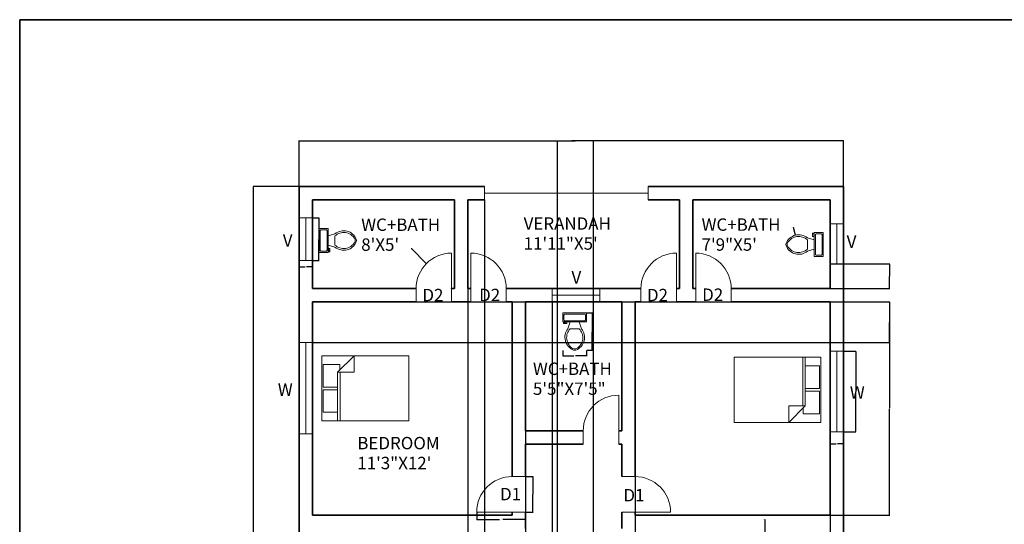
# Model space of a CAD drawing. Units: feet. Extents: x 1654 to 2985, y 1348 to 2230.
# Tile 40 of 53: x 1654 to 2320, y 1889 to 2230. Entities that reach past the tile are written whole.
import ezdxf

# ---------------------------------------------------------------- set-up
doc = ezdxf.new("R2010")
doc.units = ezdxf.units.FT
for name, color, linetype, lineweight in [('A-ANNO-DIMS', 2, 'Continuous', 18), ('A-ANNO-TEXT', 7, 'Continuous', 18), ('A-ANNO-TTLB', 7, 'Continuous', 35), ('A-AREA-IDEN', 7, 'Continuous', 18), ('A-DOOR', 3, 'Continuous', 18), ('A-FLOR-FIXT', 8, 'Continuous', 18), ('A-FURN', 8, 'Continuous', 13), ('A-GLAZ', 4, 'Continuous', 18), ('A-WALL', 7, 'Continuous', 35), ('A-WALL-OPEN', 4, 'Continuous', 18)]:
    doc.layers.add(name, color=color, linetype=linetype, lineweight=lineweight)
doc.styles.get("Standard").update_dxf_attribs({"font": 'arial.ttf'})
doc.dimstyles.get("Standard").update_dxf_attribs({"dimtxt": 0.18, "dimasz": 0.18, "dimexe": 0.18, "dimexo": 0.0625, "dimgap": 0.09, "dimtad": 0, "dimtih": 1, "dimtoh": 1, "dimdec": 4, "dimzin": 0, "dimdsep": 46, "dimtxsty": 'Standard', "dimcen": 0.09, "dimadec": 0, "dimazin": 0, "dimtfac": 1, "dimtdec": 4, "dimtofl": 0, "dimtmove": 0, "dimatfit": 3, "dimfxl": 1, "dimtolj": 1, "dimtzin": 0, "dimarcsym": 0})

# ---------------------------------------------------------------- blocks, each defined once
blk = doc.blocks.new('Toilet - top')
for p, q in [((-10, -8.5), (-8, -8.5)), ((-10, -9.5), (-10, -8.5)), ((-8, -8.5), (-8, -8)), ((-7, -8), (-7, -9.5)), ((-4, -8), (-6, -14)), ((4, -8), (6, -14)), ((9.5, -6), (9.5, -2)), ((-7, -9.5), (-10, -9.5)), ((4, -14), (-4, -14))]:
    blk.add_line(p, q)
blk.add_lwpolyline([(10.5, -8), (10.5, 0), (-10.5, 0), (-10.5, -8)], close=True)
for points in [[(-9.5, -2), (-9.5, -6)], [(8.5, -1), (-8.5, -1)], [(-8.5, -7), (8.5, -7)]]:
    blk.add_lwpolyline(points)
for centre, radius, start, end in [((-8.62, -1.88), 0.884, 81.8699, 188.1301), ((-8.62, -6.12), 0.884, 171.8699, 278.1301), ((8.62, -1.88), 0.884, 351.8699, 98.1301), ((8.62, -6.12), 0.884, 261.8699, 8.1301), ((3.52, -21.58), 12.17, 141.46911, 247.97143), ((4.2, -21.82), 11.33, 136.36773, 238.94682), ((-3.52, -21.58), 12.17, 292.02843, 38.53071), ((-4.2, -21.82), 11.33, 301.05301, 43.63209), ((0, -27.88), 4, 245.73182, 294.26817), ((0, -29), 4, 254.86053, 285.13947)]:
    blk.add_arc(centre, radius, start, end)
blk = doc.blocks.new('Bed - Queen')
for p, q in [((0, -80.00003), (0, 0)), ((0, 0), (59.99999, 0)), ((59.99999, 0), (59.99999, -80.00003)), ((7.99999, -1.2), (28.79998, -1.2)), ((7.99999, -14.4), (7.99999, -1.2)), ((28.79998, -1.2), (28.79998, -14.4)), ((31.19999, -1.2), (51.99999, -1.2)), ((31.19999, -14.4), (31.19999, -1.2)), ((51.99999, -1.2), (51.99999, -16.4)), ((0, -14.4), (44.8, -14.4)), ((44.8, -16.8), (0, -16.8)), ((59.99999, -29.6), (44.8, -14.4)), ((44.8, -14.4), (44.8, -29.6)), ((51.99999, -16.4), (46.79936, -16.4)), ((44.8, -29.6), (59.99999, -29.6)), ((59.99999, -80.00003), (0, -80.00003))]:
    blk.add_line(p, q)
blk = doc.blocks.new('DOOR-D2-SINGLE')
for p, q in [((0, 24), (0, -9)), ((-24, 0), (-24, -9))]:
    blk.add_line(p, q)
blk.add_arc((0, 0), 24, 90, 180)
blk = doc.blocks.new('DOOR-INT-SINGLE')
for p, q in [((0, 24), (9, 24)), ((-24, 0), (9, 0))]:
    blk.add_line(p, q)
blk.add_arc((0, 0), 24, 90, 180)
blk = doc.blocks.new('VENT-BATH-WEST')
for p, q in [((0, 28.76), (9, 28.76)), ((4.5, 28.76), (4.5, 0)), ((0, 0), (9, 0))]:
    blk.add_line(p, q)
blk = doc.blocks.new('OPENING-VERANDAH')
for p, q in [((0, 9), (0, 0)), ((110.69, 9), (110.69, 0)), ((0, 4.5), (110.69, 4.5))]:
    blk.add_line(p, q)
blk = doc.blocks.new('VENT-BATH-EAST')
for p, q in [((0, 27.15), (9, 27.15)), ((4.5, 27.15), (4.5, 0)), ((0, 0), (9, 0))]:
    blk.add_line(p, q)
blk = doc.blocks.new('WIN-BED-WEST')
for p, q in [((0, 61.83), (9, 61.83)), ((4.5, 61.83), (4.5, 0)), ((0, 0), (9, 0))]:
    blk.add_line(p, q)
blk = doc.blocks.new('VENT-BATH-CENTER')
for p, q in [((0, 9), (0, 0)), ((32.4, 9), (32.4, 0)), ((0, 4.5), (32.4, 4.5))]:
    blk.add_line(p, q)
blk = doc.blocks.new('WIN-BED-EAST')
for p, q in [((0, 54.45), (9, 54.45)), ((4.5, 54.45), (4.5, 0)), ((0, 0), (9, 0))]:
    blk.add_line(p, q)
blk = doc.blocks.new('*D26')
at = {"layer": 'A-ANNO-DIMS', "color": 0, "lineweight": -2, "transparency": 16777216}
for p, q in [((1963.09, 1897.19), (1963.09, 1892.12)), ((1996.09, 1897.19), (1996.09, 1892.12)), ((1963.27, 1892.3), (1978.46, 1892.3)), ((1995.91, 1892.3), (1980.72, 1892.3))]:
    blk.add_line(p, q, dxfattribs=at)
at = {"layer": 'A-ANNO-DIMS', "color": 0, "transparency": 16777216}
for points in [[(1963.27, 1892.33), (1963.27, 1892.27), (1963.09, 1892.3)], [(1995.91, 1892.33), (1995.91, 1892.27), (1996.09, 1892.3)]]:
    blk.add_solid(points, dxfattribs=at)
at = {"layer": 'Defpoints', "color": 0, "transparency": 16777216}
for p in [(1963.09, 1897.25), (1996.09, 1897.25), (1996.09, 1892.3)]:
    blk.add_point(p, dxfattribs=at)
at = {"layer": 'A-ANNO-DIMS', "color": 0, "transparency": 16777216, "insert": (1979.59, 1892.3), "char_height": 0.18, "attachment_point": 5}
blk.add_mtext('\\A1;D1 DOOR 33 TYP.', dxfattribs=at)
blk = doc.blocks.new('*D27')
at = {"layer": 'A-ANNO-DIMS', "color": 0, "lineweight": -2, "transparency": 16777216}
for p, q in [((1996.15, 1921.25), (2001.22, 1921.25)), ((2001.04, 1921.07), (2001.04, 1909.44)), ((2001.04, 1897.43), (2001.04, 1909.07)), ((1996.15, 1897.25), (2001.22, 1897.25))]:
    blk.add_line(p, q, dxfattribs=at)
at = {"layer": 'A-ANNO-DIMS', "color": 0, "transparency": 16777216}
for points in [[(2001.01, 1921.07), (2001.07, 1921.07), (2001.04, 1921.25)], [(2001.01, 1897.43), (2001.07, 1897.43), (2001.04, 1897.25)]]:
    blk.add_solid(points, dxfattribs=at)
at = {"layer": 'Defpoints', "color": 0, "transparency": 16777216}
for p in [(1996.09, 1921.25), (2001.04, 1921.25), (1996.09, 1897.25)]:
    blk.add_point(p, dxfattribs=at)
at = {"layer": 'A-ANNO-DIMS', "color": 0, "transparency": 16777216, "insert": (2001.04, 1909.25), "char_height": 0.18, "attachment_point": 5}
blk.add_mtext('\\A1;24 TYP.', dxfattribs=at)
blk = doc.blocks.new('*D34')
at = {"layer": 'A-ANNO-DIMS', "color": 0, "lineweight": -2, "transparency": 16777216}
for p, q in [((2037.43, 2031.89), (2041.34, 2031.89)), ((2041.16, 2031.71), (2041.16, 2019.43)), ((2041.16, 2006.79), (2041.16, 2019.06)), ((2037.43, 2006.61), (2041.34, 2006.61))]:
    blk.add_line(p, q, dxfattribs=at)
at = {"layer": 'A-ANNO-DIMS', "color": 0, "transparency": 16777216}
for points in [[(2041.13, 2031.71), (2041.19, 2031.71), (2041.16, 2031.89)], [(2041.13, 2006.79), (2041.19, 2006.79), (2041.16, 2006.61)]]:
    blk.add_solid(points, dxfattribs=at)
at = {"layer": 'Defpoints', "color": 0, "transparency": 16777216}
for p in [(2037.37, 2031.89), (2041.16, 2031.89), (2037.37, 2006.61)]:
    blk.add_point(p, dxfattribs=at)
at = {"layer": 'A-ANNO-DIMS', "color": 0, "transparency": 16777216, "insert": (2041.16, 2019.25), "char_height": 0.18, "attachment_point": 5}
blk.add_mtext('\\A1;WC 25 TYP.', dxfattribs=at)
blk = doc.blocks.new('*D35')
at = {"layer": 'A-ANNO-DIMS', "color": 0, "lineweight": -2, "transparency": 16777216}
for p, q in [((2021.3, 2006.54), (2021.3, 2002.63)), ((2037.37, 2006.54), (2037.37, 2002.63)), ((2021.48, 2002.81), (2028.82, 2002.81)), ((2037.19, 2002.81), (2029.86, 2002.81))]:
    blk.add_line(p, q, dxfattribs=at)
at = {"layer": 'A-ANNO-DIMS', "color": 0, "transparency": 16777216}
for points in [[(2021.48, 2002.84), (2021.48, 2002.78), (2021.3, 2002.81)], [(2037.19, 2002.84), (2037.19, 2002.78), (2037.37, 2002.81)]]:
    blk.add_solid(points, dxfattribs=at)
at = {"layer": 'Defpoints', "color": 0, "transparency": 16777216}
for p in [(2021.3, 2006.61), (2037.37, 2006.61), (2037.37, 2002.81)]:
    blk.add_point(p, dxfattribs=at)
at = {"layer": 'A-ANNO-DIMS', "color": 0, "transparency": 16777216, "insert": (2029.34, 2002.81), "char_height": 0.18, "attachment_point": 5}
blk.add_mtext('\\A1;16 TYP.', dxfattribs=at)
blk = doc.blocks.new('*D48')
at = {"layer": 'A-ANNO-DIMS', "color": 0, "lineweight": -2, "transparency": 16777216}
for p, q in [((1852.15, 2096.1), (1856.59, 2096.1)), ((1856.41, 2095.92), (1856.41, 2081.9)), ((1856.41, 2067.52), (1856.41, 2081.54)), ((1852.15, 2067.34), (1856.59, 2067.34))]:
    blk.add_line(p, q, dxfattribs=at)
at = {"layer": 'A-ANNO-DIMS', "color": 0, "transparency": 16777216}
for points in [[(1856.38, 2095.92), (1856.44, 2095.92), (1856.41, 2096.1)], [(1856.38, 2067.52), (1856.44, 2067.52), (1856.41, 2067.34)]]:
    blk.add_solid(points, dxfattribs=at)
at = {"layer": 'Defpoints', "color": 0, "transparency": 16777216}
for p in [(1852.09, 2096.1), (1856.41, 2096.1), (1852.09, 2067.34)]:
    blk.add_point(p, dxfattribs=at)
at = {"layer": 'A-ANNO-DIMS', "color": 0, "transparency": 16777216, "insert": (1856.41, 2081.72), "char_height": 0.18, "attachment_point": 5}
blk.add_mtext('\\A1;WEST VENT 29 TYP.', dxfattribs=at)
blk = doc.blocks.new('*D49')
at = {"layer": 'A-ANNO-DIMS', "color": 0, "lineweight": -2, "transparency": 16777216}
for p, q in [((1843.09, 2067.28), (1843.09, 2062.84)), ((1843.27, 2063.02), (1847.13, 2063.02)), ((1851.91, 2063.02), (1848.05, 2063.02)), ((1852.09, 2067.28), (1852.09, 2062.84))]:
    blk.add_line(p, q, dxfattribs=at)
at = {"layer": 'A-ANNO-DIMS', "color": 0, "transparency": 16777216}
for points in [[(1843.27, 2063.05), (1843.27, 2062.99), (1843.09, 2063.02)], [(1851.91, 2063.05), (1851.91, 2062.99), (1852.09, 2063.02)]]:
    blk.add_solid(points, dxfattribs=at)
at = {"layer": 'Defpoints', "color": 0, "transparency": 16777216}
for p in [(1843.09, 2067.34), (1852.09, 2067.34), (1852.09, 2063.02)]:
    blk.add_point(p, dxfattribs=at)
at = {"layer": 'A-ANNO-DIMS', "color": 0, "transparency": 16777216, "insert": (1847.59, 2063.02), "char_height": 0.18, "attachment_point": 5}
blk.add_mtext('\\A1;9 TYP.', dxfattribs=at)
blk = doc.blocks.new('*D58')
at = {"layer": 'A-ANNO-DIMS', "color": 0, "lineweight": -2, "transparency": 16777216}
for p, q in [((2211.15, 2005.94), (2219.44, 2005.94)), ((2219.26, 2005.76), (2219.26, 1978.9)), ((2219.26, 1951.67), (2219.26, 1978.53)), ((2211.15, 1951.49), (2219.44, 1951.49))]:
    blk.add_line(p, q, dxfattribs=at)
at = {"layer": 'A-ANNO-DIMS', "color": 0, "transparency": 16777216}
for points in [[(2219.23, 2005.76), (2219.29, 2005.76), (2219.26, 2005.94)], [(2219.23, 1951.67), (2219.29, 1951.67), (2219.26, 1951.49)]]:
    blk.add_solid(points, dxfattribs=at)
at = {"layer": 'Defpoints', "color": 0, "transparency": 16777216}
for p in [(2211.09, 2005.94), (2219.26, 2005.94), (2211.09, 1951.49)]:
    blk.add_point(p, dxfattribs=at)
at = {"layer": 'A-ANNO-DIMS', "color": 0, "transparency": 16777216, "insert": (2219.26, 1978.71), "char_height": 0.18, "attachment_point": 5}
blk.add_mtext('\\A1;BEDROOM E 54 TYP.', dxfattribs=at)
blk = doc.blocks.new('*D59')
at = {"layer": 'A-ANNO-DIMS', "color": 0, "lineweight": -2, "transparency": 16777216}
for p, q in [((2202.09, 1951.43), (2202.09, 1943.14)), ((2211.09, 1951.43), (2211.09, 1943.14)), ((2202.27, 1943.32), (2206.13, 1943.32)), ((2210.91, 1943.32), (2207.05, 1943.32))]:
    blk.add_line(p, q, dxfattribs=at)
at = {"layer": 'A-ANNO-DIMS', "color": 0, "transparency": 16777216}
for points in [[(2202.27, 1943.35), (2202.27, 1943.29), (2202.09, 1943.32)], [(2210.91, 1943.35), (2210.91, 1943.29), (2211.09, 1943.32)]]:
    blk.add_solid(points, dxfattribs=at)
at = {"layer": 'Defpoints', "color": 0, "transparency": 16777216}
for p in [(2202.09, 1951.49), (2211.09, 1951.49), (2211.09, 1943.32)]:
    blk.add_point(p, dxfattribs=at)
at = {"layer": 'A-ANNO-DIMS', "color": 0, "transparency": 16777216, "insert": (2206.59, 1943.32), "char_height": 0.18, "attachment_point": 5}
blk.add_mtext('\\A1;9 TYP.', dxfattribs=at)
blk = doc.blocks.new('*D76')
at = {"layer": 'A-ANNO-DIMS', "color": 0, "lineweight": -2, "transparency": 16777216}
for p, q in [((1843.09, 2117.32), (1843.09, 2148.43)), ((1843.27, 2148.25), (2026.8, 2148.25)), ((2210.91, 2148.25), (2027.38, 2148.25)), ((2211.09, 2117.32), (2211.09, 2148.43))]:
    blk.add_line(p, q, dxfattribs=at)
at = {"layer": 'A-ANNO-DIMS', "color": 0, "transparency": 16777216}
for points in [[(1843.27, 2148.28), (1843.27, 2148.22), (1843.09, 2148.25)], [(2210.91, 2148.28), (2210.91, 2148.22), (2211.09, 2148.25)]]:
    blk.add_solid(points, dxfattribs=at)
at = {"layer": 'Defpoints', "color": 0, "transparency": 16777216}
for p in [(2211.09, 2148.25), (1843.09, 2117.25), (2211.09, 2117.25)]:
    blk.add_point(p, dxfattribs=at)
at = {"layer": 'A-ANNO-DIMS', "color": 0, "transparency": 16777216, "insert": (2027.09, 2148.25), "char_height": 0.18, "attachment_point": 5}
blk.add_mtext('\\A1;368', dxfattribs=at)
blk = doc.blocks.new('*D77')
at = {"layer": 'A-ANNO-DIMS', "color": 0, "lineweight": -2, "transparency": 16777216}
for p, q in [((1843.03, 2117.25), (1811.91, 2117.25)), ((1812.09, 2117.07), (1812.09, 1841.44)), ((1812.09, 1565.43), (1812.09, 1841.07)), ((1843.03, 1565.25), (1811.91, 1565.25))]:
    blk.add_line(p, q, dxfattribs=at)
at = {"layer": 'A-ANNO-DIMS', "color": 0, "transparency": 16777216}
for points in [[(1812.06, 2117.07), (1812.12, 2117.07), (1812.09, 2117.25)], [(1812.06, 1565.43), (1812.12, 1565.43), (1812.09, 1565.25)]]:
    blk.add_solid(points, dxfattribs=at)
at = {"layer": 'Defpoints', "color": 0, "transparency": 16777216}
for p in [(1812.09, 2117.25), (1843.09, 2117.25), (1843.09, 1565.25)]:
    blk.add_point(p, dxfattribs=at)
at = {"layer": 'A-ANNO-DIMS', "color": 0, "transparency": 16777216, "insert": (1812.09, 1841.25), "char_height": 0.18, "attachment_point": 5}
blk.add_mtext('\\A1;552', dxfattribs=at)
blk = doc.blocks.new('*D80')
at = {"layer": 'A-ANNO-DIMS', "color": 0, "lineweight": -2, "transparency": 16777216}
for p, q in [((2070.09, 2039.19), (2070.09, 1534.07)), ((2202.09, 2039.19), (2202.09, 1534.07)), ((2070.27, 1534.25), (2135.81, 1534.25)), ((2201.91, 1534.25), (2136.37, 1534.25))]:
    blk.add_line(p, q, dxfattribs=at)
at = {"layer": 'A-ANNO-DIMS', "color": 0, "transparency": 16777216}
for points in [[(2070.27, 1534.28), (2070.27, 1534.22), (2070.09, 1534.25)], [(2201.91, 1534.28), (2201.91, 1534.22), (2202.09, 1534.25)]]:
    blk.add_solid(points, dxfattribs=at)
at = {"layer": 'Defpoints', "color": 0, "transparency": 16777216}
for p in [(2070.09, 2039.25), (2202.09, 2039.25), (2202.09, 1534.25)]:
    blk.add_point(p, dxfattribs=at)
at = {"layer": 'A-ANNO-DIMS', "color": 0, "transparency": 16777216, "insert": (2136.09, 1534.25), "char_height": 0.18, "attachment_point": 5}
blk.add_mtext('\\A1;132', dxfattribs=at)
blk = doc.blocks.new('*D81')
at = {"layer": 'A-ANNO-DIMS', "color": 0, "lineweight": -2, "transparency": 16777216}
for p, q in [((2202.15, 2039.25), (2242.27, 2039.25)), ((2242.09, 2039.07), (2242.09, 1967.44)), ((2242.09, 1895.43), (2242.09, 1967.07)), ((2202.15, 1895.25), (2242.27, 1895.25))]:
    blk.add_line(p, q, dxfattribs=at)
at = {"layer": 'A-ANNO-DIMS', "color": 0, "transparency": 16777216}
for points in [[(2242.06, 2039.07), (2242.12, 2039.07), (2242.09, 2039.25)], [(2242.06, 1895.43), (2242.12, 1895.43), (2242.09, 1895.25)]]:
    blk.add_solid(points, dxfattribs=at)
at = {"layer": 'Defpoints', "color": 0, "transparency": 16777216}
for p in [(2202.09, 2039.25), (2242.09, 2039.25), (2202.09, 1895.25)]:
    blk.add_point(p, dxfattribs=at)
at = {"layer": 'A-ANNO-DIMS', "color": 0, "transparency": 16777216, "insert": (2242.09, 1967.25), "char_height": 0.18, "attachment_point": 5}
blk.add_mtext('\\A1;144', dxfattribs=at)
blk = doc.blocks.new('*D88')
at = {"layer": 'A-ANNO-DIMS', "color": 0, "lineweight": -2, "transparency": 16777216}
for p, q in [((2017.77, 1661.32), (2017.77, 2148.43)), ((2017.95, 2148.25), (2029.55, 2148.25)), ((2041.9, 2148.25), (2030.3, 2148.25)), ((2042.08, 1661.32), (2042.08, 2148.43))]:
    blk.add_line(p, q, dxfattribs=at)
at = {"layer": 'A-ANNO-DIMS', "color": 0, "transparency": 16777216}
for points in [[(2017.95, 2148.28), (2017.95, 2148.22), (2017.77, 2148.25)], [(2041.9, 2148.28), (2041.9, 2148.22), (2042.08, 2148.25)]]:
    blk.add_solid(points, dxfattribs=at)
at = {"layer": 'Defpoints', "color": 0, "transparency": 16777216}
for p in [(2017.77, 2148.25), (2017.77, 1661.25), (2042.08, 1661.25)]:
    blk.add_point(p, dxfattribs=at)
at = {"layer": 'A-ANNO-DIMS', "color": 0, "transparency": 16777216, "insert": (2029.92, 2148.25), "char_height": 0.18, "attachment_point": 5}
blk.add_mtext('\\A1;24.31', dxfattribs=at)
blk = doc.blocks.new('*D92')
at = {"layer": 'A-ANNO-DIMS', "color": 0, "lineweight": -2, "transparency": 16777216}
for p, q in [((1852.15, 2039.25), (2242.27, 2039.25)), ((2242.09, 2039.07), (2242.09, 2025.79)), ((2242.09, 2012.13), (2242.09, 2025.42)), ((1852.15, 2011.95), (2242.27, 2011.95))]:
    blk.add_line(p, q, dxfattribs=at)
at = {"layer": 'A-ANNO-DIMS', "color": 0, "transparency": 16777216}
for points in [[(2242.06, 2039.07), (2242.12, 2039.07), (2242.09, 2039.25)], [(2242.06, 2012.13), (2242.12, 2012.13), (2242.09, 2011.95)]]:
    blk.add_solid(points, dxfattribs=at)
at = {"layer": 'Defpoints', "color": 0, "transparency": 16777216}
for p in [(1852.09, 2039.25), (2242.09, 2039.25), (1852.09, 2011.95)]:
    blk.add_point(p, dxfattribs=at)
at = {"layer": 'A-ANNO-DIMS', "color": 0, "transparency": 16777216, "insert": (2242.09, 2025.6), "char_height": 0.18, "attachment_point": 5}
blk.add_mtext('\\A1;27.3', dxfattribs=at)
blk = doc.blocks.new('*D94')
at = {"layer": 'A-ANNO-DIMS', "color": 0, "lineweight": -2, "transparency": 16777216}
for p, q in [((2202.15, 2064.95), (2242.27, 2064.95)), ((2242.09, 2064.77), (2242.09, 2056.78)), ((2242.09, 2048.43), (2242.09, 2056.42)), ((2202.15, 2048.25), (2242.27, 2048.25))]:
    blk.add_line(p, q, dxfattribs=at)
at = {"layer": 'A-ANNO-DIMS', "color": 0, "transparency": 16777216}
for points in [[(2242.06, 2064.77), (2242.12, 2064.77), (2242.09, 2064.95)], [(2242.06, 2048.43), (2242.12, 2048.43), (2242.09, 2048.25)]]:
    blk.add_solid(points, dxfattribs=at)
at = {"layer": 'Defpoints', "color": 0, "transparency": 16777216}
for p in [(2202.09, 2064.95), (2242.09, 2064.95), (2202.09, 2048.25)]:
    blk.add_point(p, dxfattribs=at)
at = {"layer": 'A-ANNO-DIMS', "color": 0, "transparency": 16777216, "insert": (2242.09, 2056.6), "char_height": 0.18, "attachment_point": 5}
blk.add_mtext('\\A1;16.694', dxfattribs=at)
blk = doc.blocks.new('*D97')
at = {"layer": 'A-ANNO-DIMS', "color": 0, "lineweight": -2, "transparency": 16777216}
for p, q in [((1957.09, 2108.19), (1957.09, 1534.07)), ((1968.25, 2108.19), (1968.25, 1534.07)), ((1957.27, 1534.25), (1962.22, 1534.25)), ((1968.07, 1534.25), (1963.13, 1534.25))]:
    blk.add_line(p, q, dxfattribs=at)
at = {"layer": 'A-ANNO-DIMS', "color": 0, "transparency": 16777216}
for points in [[(1957.27, 1534.28), (1957.27, 1534.22), (1957.09, 1534.25)], [(1968.07, 1534.28), (1968.07, 1534.22), (1968.25, 1534.25)]]:
    blk.add_solid(points, dxfattribs=at)
at = {"layer": 'Defpoints', "color": 0, "transparency": 16777216}
for p in [(1957.09, 2108.25), (1968.25, 2108.25), (1968.25, 1534.25)]:
    blk.add_point(p, dxfattribs=at)
at = {"layer": 'A-ANNO-DIMS', "color": 0, "transparency": 16777216, "insert": (1962.67, 1534.25), "char_height": 0.18, "attachment_point": 5}
blk.add_mtext('\\A1;11.162', dxfattribs=at)
blk = doc.blocks.new('*D101')
at = {"layer": 'A-ANNO-DIMS', "color": 0, "lineweight": -2, "transparency": 16777216}
for p, q in [((1996.09, 2039.19), (1996.09, 1534.07)), ((2014.02, 2039.19), (2014.02, 1534.07)), ((1996.27, 1534.25), (2004.6, 1534.25)), ((2013.84, 1534.25), (2005.51, 1534.25))]:
    blk.add_line(p, q, dxfattribs=at)
at = {"layer": 'A-ANNO-DIMS', "color": 0, "transparency": 16777216}
for points in [[(1996.27, 1534.28), (1996.27, 1534.22), (1996.09, 1534.25)], [(2013.84, 1534.28), (2013.84, 1534.22), (2014.02, 1534.25)]]:
    blk.add_solid(points, dxfattribs=at)
at = {"layer": 'Defpoints', "color": 0, "transparency": 16777216}
for p in [(1996.09, 2039.25), (2014.02, 2039.25), (2014.02, 1534.25)]:
    blk.add_point(p, dxfattribs=at)
at = {"layer": 'A-ANNO-DIMS', "color": 0, "transparency": 16777216, "insert": (2005.05, 1534.25), "char_height": 0.18, "attachment_point": 5}
blk.add_mtext('\\A1;17.924', dxfattribs=at)
blk = doc.blocks.new('*D104')
at = {"layer": 'A-ANNO-DIMS', "color": 0, "lineweight": -2, "transparency": 16777216}
for p, q in [((1918.76, 2075.41), (1918.94, 2075.41)), ((1918.94, 2075.41), (1928.99, 2065.35)), ((1946, 2048.25), (1946.18, 2048.25)), ((1946.09, 2048.16), (1946.09, 2048.34))]:
    blk.add_line(p, q, dxfattribs=at)
at = {"layer": 'A-ANNO-DIMS', "color": 0, "transparency": 16777216}
blk.add_solid([(1929.02, 2065.37), (1928.97, 2065.33), (1929.12, 2065.23)], dxfattribs=at)
at = {"layer": 'Defpoints', "color": 0, "transparency": 16777216}
for p in [(1929.12, 2065.23), (1946.09, 2048.25)]:
    blk.add_point(p, dxfattribs=at)
at = {"layer": 'A-ANNO-DIMS', "color": 0, "transparency": 16777216, "insert": (1918.26, 2075.41), "char_height": 0.18, "attachment_point": 5}
blk.add_mtext('\\A1;7X R24', dxfattribs=at)
blk = doc.blocks.new('*D110')
at = {"layer": 'A-ANNO-DIMS', "color": 0, "lineweight": -2, "transparency": 16777216}
for p, q in [((2157.58, 1892.24), (2157.76, 1892.24)), ((2157.76, 1892.24), (2157.76, 1875.33)), ((2157.67, 1846.66), (2157.85, 1846.66)), ((2157.76, 1846.57), (2157.76, 1846.75))]:
    blk.add_line(p, q, dxfattribs=at)
at = {"layer": 'A-ANNO-DIMS', "color": 0, "transparency": 16777216}
blk.add_solid([(2157.79, 1875.33), (2157.73, 1875.33), (2157.76, 1875.15)], dxfattribs=at)
at = {"layer": 'Defpoints', "color": 0, "transparency": 16777216}
for p in [(2157.76, 1875.15), (2157.76, 1846.66)]:
    blk.add_point(p, dxfattribs=at)
at = {"layer": 'A-ANNO-DIMS', "color": 0, "transparency": 16777216, "insert": (2156.91, 1892.24), "char_height": 0.18, "attachment_point": 5}
blk.add_mtext('\\A1;2X R28.49', dxfattribs=at)
blk = doc.blocks.new('*D112')
at = {"layer": 'A-ANNO-DIMS', "color": 0, "lineweight": -2, "transparency": 16777216}
for p, q in [((2176.87, 2089.81), (2177.05, 2089.81)), ((2177.05, 2089.81), (2178.42, 2084.58)), ((2180.74, 2075.4), (2180.92, 2075.4)), ((2180.83, 2075.31), (2180.83, 2075.49))]:
    blk.add_line(p, q, dxfattribs=at)
at = {"layer": 'A-ANNO-DIMS', "color": 0, "transparency": 16777216}
blk.add_solid([(2178.45, 2084.59), (2178.39, 2084.57), (2178.47, 2084.41)], dxfattribs=at)
at = {"layer": 'Defpoints', "color": 0, "transparency": 16777216}
for p in [(2178.47, 2084.41), (2180.83, 2075.4)]:
    blk.add_point(p, dxfattribs=at)
at = {"layer": 'A-ANNO-DIMS', "color": 0, "transparency": 16777216, "insert": (2176.15, 2089.81), "char_height": 0.18, "attachment_point": 5}
blk.add_mtext('\\A1;12X R9.311', dxfattribs=at)

msp = doc.modelspace()

# ---------------------------------------------------------------- linework, layer by layer
at = {"layer": 'A-ANNO-TTLB'}
msp.add_lwpolyline([(1654.1997, 2230.0267), (2985.175, 2230.0267), (2985.175, 1348.1324), (1654.1997, 1348.1324)], close=True, dxfattribs=at)
at = {"layer": 'A-WALL'}
for p, q in [((1843.0924, 2117.2549), (1968.2542, 2117.2549)), ((1843.0924, 2048.2549), (1843.0924, 2117.2549)), ((1843.0924, 2117.2549), (1843.0924, 1565.2549)), ((1957.0924, 2117.2549), (1968.2542, 2117.2549)), ((2078.9421, 2117.2549), (2100.0924, 2117.2549)), ((2078.9421, 2117.2549), (2211.0924, 2117.2549)), ((2109.0924, 2117.2549), (2211.0924, 2117.2549)), ((2211.0924, 2117.2549), (2211.0924, 1742.2549)), ((1852.0924, 2108.2549), (1948.0924, 2108.2549)), ((1852.0924, 2048.2549), (1852.0924, 2108.2549)), ((1948.0924, 2108.2549), (1948.0924, 2048.2549)), ((1957.0924, 2108.2549), (1957.0924, 2048.2549)), ((1957.0924, 2108.2549), (1968.2542, 2108.2549)), ((2078.9421, 2108.2549), (2100.0924, 2108.2549)), ((2100.0924, 2108.2549), (2100.0924, 2048.2549)), ((2109.0924, 2108.2549), (2109.0924, 2048.2549)), ((2109.0924, 2108.2549), (2202.0924, 2108.2549)), ((2202.0924, 2108.2549), (2202.0924, 2048.2549)), ((1922.0924, 2048.2549), (1852.0924, 2048.2549)), ((1948.0924, 2048.2549), (1946.0924, 2048.2549)), ((1959.0924, 2048.2549), (1957.0924, 2048.2549)), ((2074.0924, 2048.2549), (1983.0924, 2048.2549)), ((2100.0924, 2048.2549), (2098.0924, 2048.2549)), ((2111.0924, 2048.2549), (2109.0924, 2048.2549)), ((2202.0924, 2048.2549), (2135.0924, 2048.2549)), ((1852.0924, 2039.2549), (1852.0924, 1895.2549)), ((1922.0924, 2039.2549), (1852.0924, 2039.2549)), ((1959.0924, 2039.2549), (1946.0924, 2039.2549)), ((1959.0924, 2039.2549), (1957.0924, 2039.2549)), ((1987.0924, 2039.2549), (1983.0924, 2039.2549)), ((1987.0924, 2039.2549), (1983.0924, 2039.2549)), ((1987.0924, 1921.2549), (1987.0924, 2039.2549)), ((2061.0924, 2039.2549), (1996.0924, 2039.2549)), ((1996.0924, 1952.2549), (1996.0924, 2039.2549)), ((2061.0924, 1952.2549), (2061.0924, 2039.2549)), ((2074.0924, 2039.2549), (2070.0924, 2039.2549)), ((2070.0924, 1921.2549), (2070.0924, 2039.2549)), ((2111.0924, 2039.2549), (2098.0924, 2039.2549)), ((2111.0924, 2039.2549), (2109.0924, 2039.2549)), ((2202.0924, 2039.2549), (2135.0924, 2039.2549)), ((2202.0924, 2039.2549), (2135.0924, 2039.2549)), ((2202.0924, 2039.2549), (2202.0924, 1895.2549)), ((2211.0924, 2039.2549), (2211.0924, 1895.2549)), ((2035.0924, 1952.2549), (1996.0924, 1952.2549)), ((2061.0924, 1952.2549), (2059.0924, 1952.2549)), ((1996.0924, 1921.2549), (1996.0924, 1943.2549)), ((2035.0924, 1943.2549), (1996.0924, 1943.2549)), ((2061.0924, 1943.2549), (2059.0924, 1943.2549)), ((2061.0924, 1921.2549), (2061.0924, 1943.2549)), ((1987.0924, 1895.2549), (1987.0924, 1897.2549)), ((1996.0924, 1886.2549), (1996.0924, 1897.2549)), ((2061.0924, 1895.2549), (2061.0924, 1897.2549)), ((2070.0924, 1895.2549), (2070.0924, 1897.2549)), ((1852.0924, 1895.2549), (1987.0924, 1895.2549)), ((2061.0924, 1895.2549), (2061.0924, 1886.2549)), ((2202.0924, 1895.2549), (2070.0924, 1895.2549))]:
    msp.add_line(p, q, dxfattribs=at)

# ---------------------------------------------------------------- block references
at = {"layer": 'A-DOOR'}
for name, p in [('DOOR-D2-SINGLE', (1946.0924, 2048.2549)), ('DOOR-D2-SINGLE', (2098.0924, 2048.2549)), ('DOOR-INT-SINGLE', (1987.0924, 1897.2549))]:
    msp.add_blockref(name, p, dxfattribs=at)
at = {"layer": 'A-DOOR', "extrusion": (0, 0, -1), "zscale": -1}
for name, p in [('DOOR-D2-SINGLE', (-1959.0924, 2048.2549)), ('DOOR-D2-SINGLE', (-2111.0924, 2048.2549)), ('DOOR-INT-SINGLE', (-2070.0924, 1897.2549))]:
    msp.add_blockref(name, p, dxfattribs=at)
at = {"layer": 'A-DOOR', "extrusion": (0, 0, -1), "zscale": -1, "rotation": 270.0000000000007}
msp.add_blockref('DOOR-INT-SINGLE', (-2059.0924, 1952.2549), dxfattribs=at)
at = {"layer": 'A-FLOR-FIXT', "xscale": 0.7651522138144634, "yscale": 0.7651522138144634, "zscale": 0.7651522138144634}
for p, rotation in [((1856.5679, 2080.7996), 90), ((2197.3441, 2078.0929), 270)]:
    msp.add_blockref('Toilet - top', p, dxfattribs=dict(at, rotation=rotation))
msp.add_blockref('Toilet - top', (2029.337, 2031.8905), dxfattribs=at)
at = {"layer": 'A-FURN', "xscale": 0.7339343441631778, "yscale": 0.7339343441631778, "zscale": 0.7339343441631778}
for p, rotation in [((1858.4494, 1958.8411), 90), ((2195.7465, 2001.9019), 270)]:
    msp.add_blockref('Bed - Queen', p, dxfattribs=dict(at, rotation=rotation))
at = {"layer": 'A-GLAZ'}
for name, p in [('VENT-BATH-WEST', (1843.092, 2067.339)), ('VENT-BATH-EAST', (2202.092, 2064.949)), ('VENT-BATH-CENTER', (2014.016, 2039.255)), ('WIN-BED-WEST', (1843.092, 1950.122)), ('WIN-BED-EAST', (2202.092, 1951.488))]:
    msp.add_blockref(name, p, dxfattribs=at)
at = {"layer": 'A-WALL-OPEN'}
msp.add_blockref('OPENING-VERANDAH', (1968.254, 2108.255), dxfattribs=at)

# ---------------------------------------------------------------- texts
at = {"layer": 'A-ANNO-TEXT'}
for s, height, p in [('V', 8.3811, (1832.0255, 2076.6892)), ('V', 8.3811, (2213.1305, 2075.7989)), ('V', 8.3811, (2027.1443, 2051.7341)), ('D2', 8.38114, (1926.4011, 2039.7278)), ('D2', 8.38114, (1964.7393, 2039.8017)), ('D2', 8.38114, (2078.1697, 2039.7473)), ('D2', 8.38114, (2115.4692, 2039.9826)), ('W', 8.3811, (1828.6747, 1975.7867)), ('W', 8.3811, (2215.2856, 1973.858)), ('D1', 8.38114, (1978.8669, 1905.2296)), ('D1', 8.38114, (2062.2606, 1904.4938))]:
    msp.add_text(s, height=height, dxfattribs=at).set_placement(p)
at = {"layer": 'A-AREA-IDEN'}
for s, p in [('VERANDAH', (1994.8342, 2088.049)), ('WC+BATH', (1885.0398, 2087.2734)), ('WC+BATH', (2115.0983, 2087.3504)), ('11\'11"X5\'', (1994.8342, 2074.5854)), ("8'X5'", (1885.0398, 2073.8098)), ('7\'9"X5\'', (2115.0983, 2073.8868)), ('WC+BATH', (2001.1048, 1989.9081)), ('5\'5"X7\'5"', (2001.1048, 1976.4445)), ('BEDROOM', (1882.4007, 1939.6855)), ('11\'3"X12\'', (1882.4007, 1926.222))]:
    msp.add_text(s, height=8.38114, dxfattribs=at).set_placement(p)

# ---------------------------------------------------------------- dimensions: what is measured, and where the dimension line sits
at = {"layer": 'A-ANNO-DIMS'}
for base, p1, p2, override, picture, middle in [((2211.0924, 2148.2549), (1843.0924, 2117.2549), (2211.0924, 2117.2549), {"dimdec": 0, "dimlfac": 1, "dimrnd": 0, "dimzin": 0, "dimdsep": 46, "dimlunit": 2}, '*D76', (2027.0924, 2148.2549)), ((2017.7694, 2148.2549), (2042.0798, 1661.2549), (2017.7694, 1661.2549), {"dimdec": 2, "dimlfac": 1, "dimrnd": 0, "dimzin": 0, "dimdsep": 46, "dimlunit": 2}, '*D88', (2029.9246, 2148.2549)), ((1968.2542, 1534.2549), (1957.0924, 2108.2549), (1968.2542, 2108.2549), {"dimdec": 3, "dimlfac": 1, "dimrnd": 0, "dimzin": 0, "dimdsep": 46, "dimlunit": 2}, '*D97', (1962.6733, 1534.2549)), ((2014.016, 1534.2549), (1996.0924, 2039.2549), (2014.016, 2039.2549), {"dimdec": 3, "dimlfac": 1, "dimrnd": 0, "dimzin": 0, "dimdsep": 46, "dimlunit": 2}, '*D101', (2005.0542, 1534.2549)), ((2202.0924, 1534.2549), (2070.0924, 2039.2549), (2202.0924, 2039.2549), {"dimdec": 0, "dimlfac": 1, "dimrnd": 0, "dimzin": 0, "dimdsep": 46, "dimlunit": 2}, '*D80', (2136.0924, 1534.2549))]:
    dim = msp.add_linear_dim(base=base, p1=p1, p2=p2, dimstyle='Standard', override=override, dxfattribs=at)
    dim.commit()
    dim.dimension.update_dxf_attribs({"geometry": picture, "text_midpoint": middle})
for base, p1, p2, override, picture, middle in [((1812.0924, 2117.2549), (1843.0924, 1565.2549), (1843.0924, 2117.2549), {"dimdec": 0, "dimlfac": 1, "dimrnd": 0, "dimzin": 0, "dimdsep": 46, "dimlunit": 2}, '*D77', (1812.0924, 1841.2549)), ((2242.0924, 2064.9486), (2202.0924, 2048.2549), (2202.0924, 2064.9486), {"dimdec": 3, "dimlfac": 1, "dimrnd": 0, "dimzin": 0, "dimdsep": 46, "dimlunit": 2}, '*D94', (2242.0924, 2056.6018)), ((2242.0924, 2039.2549), (1852.0924, 2011.9524), (1852.0924, 2039.2549), {"dimdec": 1, "dimlfac": 1, "dimrnd": 0, "dimzin": 0, "dimdsep": 46, "dimlunit": 2}, '*D92', (2242.0924, 2025.6037)), ((2242.0924, 2039.2549), (2202.0924, 1895.2549), (2202.0924, 2039.2549), {"dimdec": 0, "dimlfac": 1, "dimrnd": 0, "dimzin": 0, "dimdsep": 46, "dimlunit": 2}, '*D81', (2242.0924, 1967.2549))]:
    dim = msp.add_linear_dim(base=base, p1=p1, p2=p2, angle=90, dimstyle='Standard', override=override, dxfattribs=at)
    dim.commit()
    dim.dimension.update_dxf_attribs({"geometry": picture, "text_midpoint": middle})
for base, p1, p2, text, picture, middle in [((1856.4069, 2096.1027), (1852.0924, 2067.3393), (1852.0924, 2096.1027), 'WEST VENT <> TYP.', '*D48', (1856.4069, 2081.721)), ((2041.1639, 2031.8905), (2037.3711, 2006.6051), (2037.3711, 2031.8905), 'WC <> TYP.', '*D34', (2041.1639, 2019.2478)), ((2219.2599, 2005.937), (2211.0924, 1951.4875), (2211.0924, 2005.937), 'BEDROOM E <> TYP.', '*D58', (2219.2599, 1978.7123)), ((2001.0424, 1921.2549), (1996.0924, 1897.2549), (1996.0924, 1921.2549), '<> TYP.', '*D27', (2001.0424, 1909.2549))]:
    dim = msp.add_linear_dim(base=base, p1=p1, p2=p2, angle=90, text=text, dimstyle='Standard', override={"dimdec": 0, "dimlfac": 1, "dimrnd": 0, "dimzin": 0, "dimdsep": 46, "dimlunit": 2}, dxfattribs=at)
    dim.commit()
    dim.dimension.update_dxf_attribs({"geometry": picture, "text_midpoint": middle})
for center, mpoint, text, override, picture, middle in [((2180.8318, 2075.3999), (2178.4659, 2084.4055), '12X <>', {"dimdec": 3, "dimlfac": 1, "dimrnd": 0, "dimzin": 0, "dimdsep": 46, "dimlunit": 2}, '*D112', (2176.149, 2089.8088)), ((1946.0924, 2048.2549), (1929.1217, 2065.2253), '7X <>', {"dimdec": 0, "dimlfac": 1, "dimrnd": 0, "dimzin": 0, "dimdsep": 46, "dimlunit": 2}, '*D104', (1918.2619, 2075.4075)), ((2157.7631, 1846.6582), (2157.763, 1875.1496), '2X <>', {"dimdec": 2, "dimlfac": 1, "dimrnd": 0, "dimzin": 0, "dimdsep": 46, "dimlunit": 2}, '*D110', (2156.908, 1892.2445))]:
    dim = msp.add_radius_dim(center=center, mpoint=mpoint, text=text, dimstyle='Standard', override=override, dxfattribs=at)
    dim.commit()
    dim.dimension.update_dxf_attribs({"geometry": picture, "text_midpoint": middle, "dimtype": 164})
for base, p1, p2, text, picture, middle in [((1852.0924, 2063.0248), (1843.0924, 2067.3393), (1852.0924, 2067.3393), '<> TYP.', '*D49', (1847.5924, 2063.0248)), ((2037.3711, 2002.8123), (2021.3029, 2006.6051), (2037.3711, 2006.6051), '<> TYP.', '*D35', (2029.337, 2002.8123)), ((2211.0924, 1943.3201), (2202.0924, 1951.4875), (2211.0924, 1951.4875), '<> TYP.', '*D59', (2206.5924, 1943.3201)), ((1996.0924, 1892.3049), (1963.0924, 1897.2549), (1996.0924, 1897.2549), 'D1 DOOR <> TYP.', '*D26', (1979.5924, 1892.3049))]:
    dim = msp.add_linear_dim(base=base, p1=p1, p2=p2, text=text, dimstyle='Standard', override={"dimdec": 0, "dimlfac": 1, "dimrnd": 0, "dimzin": 0, "dimdsep": 46, "dimlunit": 2}, dxfattribs=at)
    dim.commit()
    dim.dimension.update_dxf_attribs({"geometry": picture, "text_midpoint": middle})

doc.saveas('drawing.dxf')
